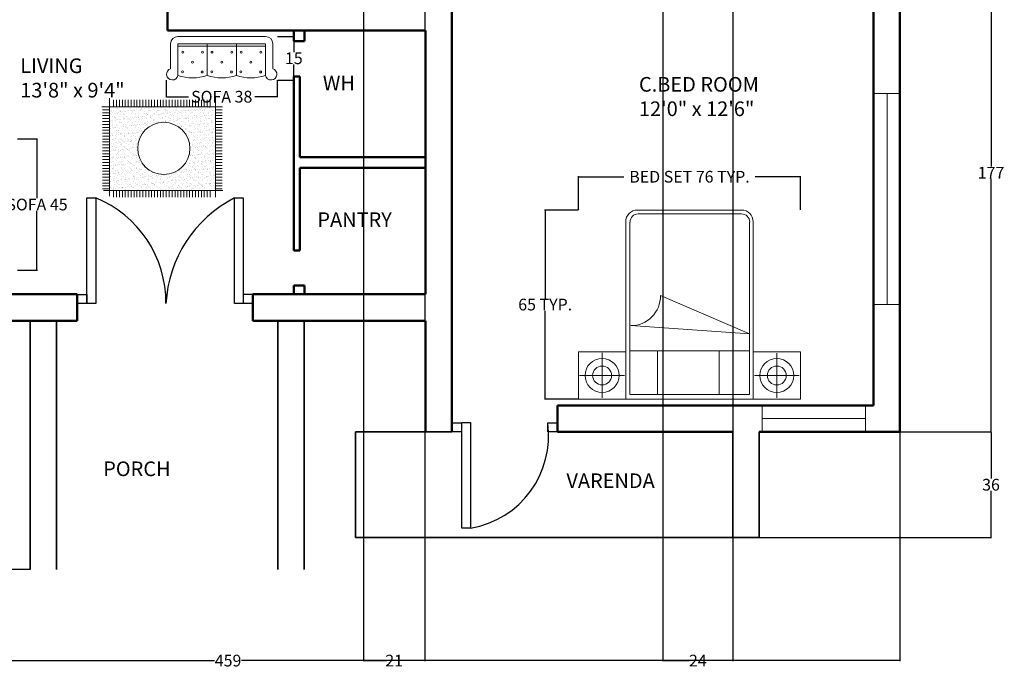
# Model space of a CAD drawing. Units: inches. Extents: x 870 to 1431, y 383 to 1070.
# Tile 2 of 9: x 1091 to 1428, y 383 to 604. Entities that reach past the tile are written whole.
import ezdxf
from ezdxf.lldxf.tags import DXFTag

# ---------------------------------------------------------------- set-up
doc = ezdxf.new("R2010")
doc.units = ezdxf.units.IN
doc.header["$MEASUREMENT"] = 0
for name, color, linetype, lineweight in [('A-ANNO-DIMS', 2, 'Continuous', 18), ('A-AREA-IDEN', 7, 'Continuous', 25), ('A-DOOR', 3, 'Continuous', 25), ('A-FLOR-EXTR', 7, 'Continuous', 35), ('A-FLOR-PATT', 252, 'Continuous', 13), ('A-FLOR-PORC', 7, 'HOT_WATER_SUPPLY', 35), ('A-FURN', 8, 'Continuous', 18), ('A-GLAZ', 4, 'Continuous', 18), ('A-WALL', 7, 'Continuous', 50)]:
    doc.layers.add(name, color=color, linetype=linetype, lineweight=lineweight)
doc.styles.get("Standard").update_dxf_attribs({"font": 'arial.ttf'})
tags = doc.linetypes.add('HOT_WATER_SUPPLY', pattern='A,0.5,-0.2,["HW",Standard,S=0.1,R=0,X=-0.1,Y=-0.05],-0.2', length=0.9).pattern_tags.tags
tags[6] = DXFTag(74, 10)
doc.dimstyles.get("Standard").update_dxf_attribs({"dimtxt": 4, "dimasz": 0.18, "dimexe": 0.18, "dimexo": 0.0625, "dimgap": 0.09, "dimtad": 0, "dimtih": 1, "dimtoh": 1, "dimdec": 0, "dimrnd": 6, "dimzin": 0, "dimdsep": 46, "dimlunit": 3, "dimtxsty": 'Standard', "dimcen": 0.09, "dimadec": 0, "dimazin": 0, "dimtfac": 1, "dimtdec": 0, "dimtofl": 0, "dimtmove": 0, "dimatfit": 3, "dimfxl": 1, "dimtolj": 1, "dimtzin": 0, "dimarcsym": 0})

# ---------------------------------------------------------------- blocks, each defined once
blk = doc.blocks.new('A$C65997121')
for p, q in [((0, 1.5, -0.169), (0, 2, -0.169)), ((0, 2, -0.169), (0.5, 2, -0.169)), ((0, 1.5, -0.169), (0, 2, -0.169)), ((0, 2, -0.169), (0.5, 2, -0.169)), ((0.25, 1.75, -0.169), (0.25, 1.988, -0.169)), ((0.5, 2, -0.169), (1.755, 2, -0.169)), ((0.5, 2, -0.169), (1.512, 2, -0.169)), ((0.5, 2, -0.169), (1.512, 2, -0.169)), ((0.5, 0.125, -0.169), (0.5, 2, -0.169)), ((0.5, 2, -0.169), (0.5, 1.5, -0.169)), ((1.512, 2, -0.169), (2.35, 2, -0.169)), ((1.512, 2, -0.169), (2.35, 2, -0.169)), ((1.85, 2, -0.169), (2.35, 2, -0.169)), ((1.85, 1.5, -0.169), (1.85, 2, -0.169)), ((2.1, 1.75, -0.169), (2.1, 1.988, -0.169)), ((2.35, 2, -0.169), (2.35, 1.5, -0.169)), ((2.35, 2, -0.169), (2.35, 1.5, -0.169)), ((2.35, 2, -0.169), (2.35, 1.5, -0.169)), ((0.538, 1.488, -0.169), (0.538, 1.952, -0.169)), ((0.538, 1.952, -0.169), (1.805, 1.952, -0.169)), ((0.86, 1.952, -0.169), (0.86, 1.488, -0.169)), ((1.512, 1.952, -0.169), (1.512, 1.488, -0.169)), ((1.805, 1.952, -0.169), (1.805, 1.488, -0.169)), ((0.25, 1.75, -0.169), (0.012, 1.75, -0.169)), ((0.25, 1.75, -0.169), (0.25, 1.512, -0.169)), ((0.25, 1.75, -0.169), (0.488, 1.75, -0.169)), ((2.1, 1.75, -0.169), (1.862, 1.75, -0.169)), ((2.1, 1.75, -0.169), (2.338, 1.75, -0.169)), ((2.1, 1.75, -0.169), (2.1, 1.512, -0.169)), ((0.5, 1.5, -0.169), (0, 1.5, -0.169)), ((0.5, 1.5, -0.169), (0, 1.5, -0.169)), ((0.5, 0.125, -0.169), (0.5, 1.5, -0.169)), ((1.805, 1.488, -0.169), (0.538, 1.488, -0.169)), ((0.538, 0.128, -0.169), (0.538, 1.488, -0.169)), ((1.805, 1.488, -0.169), (1.805, 0.128, -0.169)), ((2.35, 1.5, -0.169), (1.85, 1.5, -0.169)), ((2.35, 1.5, -0.169), (1.85, 1.5, -0.169)), ((1.85, 1.5, -0.169), (1.85, 0.125, -0.169)), ((2.35, 1.5, -0.169), (1.85, 1.5, -0.169)), ((1.85, 1.5, -0.169), (1.85, 0.125, -0.169)), ((1.483, 0.905, -0.506), (0.538, 1.31, -0.506)), ((0.538, 1.31, -0.506), (1.797, 1.222, -0.506)), ((1.717, 0.04, -0.169), (0.625, 0.04, -0.169)), ((1.725, 0, -0.169), (0.625, 0, -0.169)), ((1.725, 0, -0.169), (0.625, 0, -0.169))]:
    blk.add_line(p, q)
for centre, radius in [((0.25, 1.75, -0.169), 0.18), ((2.1, 1.75, -0.169), 0.18), ((0.25, 1.75, -0.169), 0.1), ((2.1, 1.75, -0.169), 0.1)]:
    blk.add_circle(centre, radius)
for centre, radius, start, end in [((1.793, 0.911, -0.506), 0.311, 89.3268, 181.1229), ((0.625, 0.125, -0.169), 0.125, 179.9939, 269.9939), ((0.625, 0.125, -0.169), 0.125, 179.9939, 269.9939), ((0.625, 0.128, -0.169), 0.0875, 179.9939, 269.9939), ((1.717, 0.128, -0.169), 0.0875, 269.9939, 359.9939), ((1.725, 0.125, -0.169), 0.125, 269.9939, 359.9939), ((1.725, 0.125, -0.169), 0.125, 269.9939, 359.9939)]:
    blk.add_arc(centre, radius, start, end)
blk = doc.blocks.new('A$C4BF50411')
for p, q in [((0.23, 0.89, -342.513), (2.03, 0.89, -342.513)), ((0.08, 0.74, -342.513), (0.08, 0.228, -342.513)), ((0.23, 0.09, -342.513), (0.23, 0.74, -342.513)), ((0.23, 0.74, -342.513), (2.03, 0.74, -342.513)), ((0.23, 0.69, -342.513), (2.03, 0.69, -342.513)), ((0.83, 0.09, -342.513), (0.83, 0.74, -342.513)), ((1.43, 0.74, -342.513), (1.43, 0.09, -342.513)), ((2.03, 0.74, -342.513), (2.03, 0.09, -342.513)), ((2.18, 0.74, -342.513), (2.18, 0.228, -342.513))]:
    blk.add_line(p, q)
for centre in [(0.33, 0.57, -342.513), (0.735, 0.565, -342.513), (0.93, 0.57, -342.513), (1.335, 0.565, -342.513), (1.53, 0.57, -342.513), (1.935, 0.565, -342.513), (0.53, 0.365, -342.513), (1.13, 0.365, -342.513), (1.73, 0.365, -342.513), (0.325, 0.165, -342.513), (0.73, 0.16, -342.513), (0.925, 0.165, -342.513), (1.33, 0.16, -342.513), (1.525, 0.165, -342.513), (1.93, 0.16, -342.513)]:
    blk.add_circle(centre, 0.02)
for centre, radius, start, end in [((0.23, 0.74, -342.513), 0.15, 90, 180), ((2.03, 0.74, -342.513), 0.15, 0, 90), ((0.115, 0.115, -342.513), 0.118, 107.205, 347.5934), ((2.145, 0.115, -342.513), 0.118, 192.4066, 72.795), ((0.53, 0.938, -342.513), 0.9, 250.5288, 289.4712), ((1.13, 0.938, -342.513), 0.9, 250.5288, 289.4712), ((1.73, 0.938, -342.513), 0.9, 250.5288, 289.4712)]:
    blk.add_arc(centre, radius, start, end)
blk = doc.blocks.new('WIN-72IN')
blk.add_line((4.72, 72), (4.72, 0))
blk.add_lwpolyline([(0, 72), (9, 72), (9, 0), (0, 0)], close=True)
blk = doc.blocks.new('WIN-BATH-35IN')
blk.add_line((4.73, 35.25), (4.73, 0))
blk.add_lwpolyline([(0, 0), (0, 35.25), (9, 35.25), (9, 0)], close=True)
blk = doc.blocks.new('*D107')
at = {"layer": 'A-ANNO-DIMS', "color": 0, "lineweight": -2, "transparency": 16777216}
for p, q in [((1282.02, 539.3), (1282.02, 550.79)), ((1282.2, 550.61), (1297.47, 550.61)), ((1357.67, 550.61), (1342.4, 550.61)), ((1357.85, 539.29), (1357.85, 550.79))]:
    blk.add_line(p, q, dxfattribs=at)
at = {"layer": 'A-ANNO-DIMS', "color": 0, "transparency": 16777216}
for points in [[(1282.2, 550.64), (1282.2, 550.58), (1282.02, 550.61)], [(1357.67, 550.64), (1357.67, 550.58), (1357.85, 550.61)]]:
    blk.add_solid(points, dxfattribs=at)
at = {"layer": 'Defpoints', "color": 0, "transparency": 16777216}
for p in [(1282.02, 550.61), (1282.02, 539.24), (1357.85, 539.23)]:
    blk.add_point(p, dxfattribs=at)
at = {"layer": 'A-ANNO-DIMS', "color": 0, "transparency": 16777216, "insert": (1319.94, 550.61), "char_height": 4, "attachment_point": 5}
blk.add_mtext('\\A1;BED SET 76 TYP.', dxfattribs=at)
blk = doc.blocks.new('*D108')
at = {"layer": 'A-ANNO-DIMS', "color": 0, "lineweight": -2, "transparency": 16777216}
for p, q in [((1281.96, 539.24), (1270.46, 539.24)), ((1270.64, 539.06), (1270.64, 509.1)), ((1270.64, 474.88), (1270.64, 504.84)), ((1281.95, 474.7), (1270.46, 474.7))]:
    blk.add_line(p, q, dxfattribs=at)
at = {"layer": 'A-ANNO-DIMS', "color": 0, "transparency": 16777216}
for points in [[(1270.61, 539.06), (1270.67, 539.06), (1270.64, 539.24)], [(1270.61, 474.88), (1270.67, 474.88), (1270.64, 474.7)]]:
    blk.add_solid(points, dxfattribs=at)
at = {"layer": 'Defpoints', "color": 0, "transparency": 16777216}
for p in [(1282.02, 539.24), (1270.64, 474.7), (1282.01, 474.7)]:
    blk.add_point(p, dxfattribs=at)
at = {"layer": 'A-ANNO-DIMS', "color": 0, "transparency": 16777216, "insert": (1270.64, 506.97), "char_height": 4, "attachment_point": 5}
blk.add_mtext('\\A1;65 TYP.', dxfattribs=at)
blk = doc.blocks.new('*D113')
at = {"layer": 'A-ANNO-DIMS', "color": 0, "lineweight": -2, "transparency": 16777216}
for p, q in [((1141.19, 583.55), (1141.19, 577.75)), ((1179.08, 583.55), (1179.08, 577.75)), ((1141.37, 577.93), (1148.8, 577.93)), ((1178.9, 577.93), (1171.47, 577.93))]:
    blk.add_line(p, q, dxfattribs=at)
at = {"layer": 'A-ANNO-DIMS', "color": 0, "transparency": 16777216}
for points in [[(1141.37, 577.96), (1141.37, 577.9), (1141.19, 577.93)], [(1178.9, 577.96), (1178.9, 577.9), (1179.08, 577.93)]]:
    blk.add_solid(points, dxfattribs=at)
at = {"layer": 'Defpoints', "color": 0, "transparency": 16777216}
for p in [(1141.19, 583.61), (1179.08, 583.61), (1179.08, 577.93)]:
    blk.add_point(p, dxfattribs=at)
at = {"layer": 'A-ANNO-DIMS', "color": 0, "transparency": 16777216, "insert": (1160.13, 577.93), "char_height": 4, "attachment_point": 5}
blk.add_mtext('\\A1;SOFA 38', dxfattribs=at)
blk = doc.blocks.new('*D114')
at = {"layer": 'A-ANNO-DIMS', "color": 0, "lineweight": -2, "transparency": 16777216}
for p, q in [((1179.14, 598.49), (1184.94, 598.49)), ((1184.76, 598.31), (1184.76, 593.18)), ((1184.76, 583.79), (1184.76, 588.92)), ((1179.14, 583.61), (1184.94, 583.61))]:
    blk.add_line(p, q, dxfattribs=at)
at = {"layer": 'A-ANNO-DIMS', "color": 0, "transparency": 16777216}
for points in [[(1184.73, 598.31), (1184.79, 598.31), (1184.76, 598.49)], [(1184.73, 583.79), (1184.79, 583.79), (1184.76, 583.61)]]:
    blk.add_solid(points, dxfattribs=at)
at = {"layer": 'Defpoints', "color": 0, "transparency": 16777216}
for p in [(1179.08, 598.49), (1184.76, 598.49), (1179.08, 583.61)]:
    blk.add_point(p, dxfattribs=at)
at = {"layer": 'A-ANNO-DIMS', "color": 0, "transparency": 16777216, "insert": (1184.76, 591.05), "char_height": 4, "attachment_point": 5}
blk.add_mtext('\\A1;15', dxfattribs=at)
blk = doc.blocks.new('*D115')
at = {"layer": 'A-ANNO-DIMS', "color": 0, "lineweight": -2, "transparency": 16777216}
for p, q in [((1090.35, 563.55), (1097.19, 563.55)), ((1097.01, 563.37), (1097.01, 543.29)), ((1097.01, 518.89), (1097.01, 538.97)), ((1090.35, 518.71), (1097.19, 518.71))]:
    blk.add_line(p, q, dxfattribs=at)
at = {"layer": 'A-ANNO-DIMS', "color": 0, "transparency": 16777216}
for points in [[(1096.98, 563.37), (1097.04, 563.37), (1097.01, 563.55)], [(1096.98, 518.89), (1097.04, 518.89), (1097.01, 518.71)]]:
    blk.add_solid(points, dxfattribs=at)
at = {"layer": 'Defpoints', "color": 0, "transparency": 16777216}
for p in [(1090.29, 563.55), (1097.01, 563.55), (1090.29, 518.71)]:
    blk.add_point(p, dxfattribs=at)
at = {"layer": 'A-ANNO-DIMS', "color": 0, "transparency": 16777216, "insert": (1097.01, 541.13), "char_height": 4, "attachment_point": 5}
blk.add_mtext('\\A1;SOFA 45', dxfattribs=at)
blk = doc.blocks.new('*D125')
at = {"layer": 'A-ANNO-DIMS', "color": 0, "lineweight": -2, "transparency": 16777216}
for p, q in [((1391.79, 463.41), (1391.79, 385.26)), ((932.79, 427.41), (932.79, 385.26)), ((932.97, 385.44), (1157.7, 385.44)), ((1391.61, 385.44), (1166.88, 385.44))]:
    blk.add_line(p, q, dxfattribs=at)
at = {"layer": 'A-ANNO-DIMS', "color": 0, "transparency": 16777216}
for points in [[(932.97, 385.47), (932.97, 385.41), (932.79, 385.44)], [(1391.61, 385.47), (1391.61, 385.41), (1391.79, 385.44)]]:
    blk.add_solid(points, dxfattribs=at)
at = {"layer": 'Defpoints', "color": 0, "transparency": 16777216}
for p in [(1391.79, 463.48), (932.79, 427.48), (1391.79, 385.44)]:
    blk.add_point(p, dxfattribs=at)
at = {"layer": 'A-ANNO-DIMS', "color": 0, "transparency": 16777216, "insert": (1162.29, 385.44), "char_height": 4, "attachment_point": 5}
blk.add_mtext('\\A1;459', dxfattribs=at)
blk = doc.blocks.new('*D126')
at = {"layer": 'A-ANNO-DIMS', "color": 0, "lineweight": -2, "transparency": 16777216}
for p, q in [((1168.73, 1009.48), (876.24, 1009.48)), ((876.42, 1009.3), (876.42, 715.17)), ((876.42, 416.77), (876.42, 710.9)), ((1094.63, 416.59), (876.24, 416.59))]:
    blk.add_line(p, q, dxfattribs=at)
at = {"layer": 'A-ANNO-DIMS', "color": 0, "transparency": 16777216}
for points in [[(876.39, 1009.3), (876.45, 1009.3), (876.42, 1009.48)], [(876.39, 416.77), (876.45, 416.77), (876.42, 416.59)]]:
    blk.add_solid(points, dxfattribs=at)
at = {"layer": 'Defpoints', "color": 0, "transparency": 16777216}
for p in [(876.42, 1009.48), (1168.79, 1009.48), (1094.7, 416.59)]:
    blk.add_point(p, dxfattribs=at)
at = {"layer": 'A-ANNO-DIMS', "color": 0, "transparency": 16777216, "insert": (876.42, 713.03), "char_height": 4, "attachment_point": 5}
blk.add_mtext('\\A1;592.9', dxfattribs=at)
blk = doc.blocks.new('*D134')
at = {"layer": 'A-ANNO-DIMS', "color": 0, "lineweight": -2, "transparency": 16777216}
for p, q in [((1391.85, 640.48), (1423.14, 640.48)), ((1422.96, 640.3), (1422.96, 554.08)), ((1422.96, 463.66), (1422.96, 549.88)), ((1391.85, 463.48), (1423.14, 463.48))]:
    blk.add_line(p, q, dxfattribs=at)
at = {"layer": 'A-ANNO-DIMS', "color": 0, "transparency": 16777216}
for points in [[(1422.93, 640.3), (1422.99, 640.3), (1422.96, 640.48)], [(1422.93, 463.66), (1422.99, 463.66), (1422.96, 463.48)]]:
    blk.add_solid(points, dxfattribs=at)
at = {"layer": 'Defpoints', "color": 0, "transparency": 16777216}
for p in [(1391.79, 640.48), (1391.79, 463.48), (1422.96, 463.48)]:
    blk.add_point(p, dxfattribs=at)
at = {"layer": 'A-ANNO-DIMS', "color": 0, "transparency": 16777216, "insert": (1422.96, 551.98), "char_height": 4, "attachment_point": 5}
blk.add_mtext('\\A1;177', dxfattribs=at)
blk = doc.blocks.new('*D135')
at = {"layer": 'A-ANNO-DIMS', "color": 0, "lineweight": -2, "transparency": 16777216}
for p, q in [((1343.85, 463.48), (1423.14, 463.48)), ((1422.96, 463.3), (1422.96, 447.61)), ((1422.96, 427.66), (1422.96, 443.34)), ((1343.85, 427.48), (1423.14, 427.48))]:
    blk.add_line(p, q, dxfattribs=at)
at = {"layer": 'A-ANNO-DIMS', "color": 0, "transparency": 16777216}
for points in [[(1422.93, 463.3), (1422.99, 463.3), (1422.96, 463.48)], [(1422.93, 427.66), (1422.99, 427.66), (1422.96, 427.48)]]:
    blk.add_solid(points, dxfattribs=at)
at = {"layer": 'Defpoints', "color": 0, "transparency": 16777216}
for p in [(1343.79, 463.48), (1422.96, 463.48), (1343.79, 427.48)]:
    blk.add_point(p, dxfattribs=at)
at = {"layer": 'A-ANNO-DIMS', "color": 0, "transparency": 16777216, "insert": (1422.96, 445.48), "char_height": 4, "attachment_point": 5}
blk.add_mtext('\\A1;36', dxfattribs=at)
blk = doc.blocks.new('*D136')
at = {"layer": 'A-ANNO-DIMS', "color": 0, "lineweight": -2, "transparency": 16777216}
for p, q in [((1208.53, 986.13), (1208.53, 385.26)), ((1229.53, 986.13), (1229.53, 385.26)), ((1208.71, 385.44), (1216.43, 385.44)), ((1229.35, 385.44), (1221.64, 385.44))]:
    blk.add_line(p, q, dxfattribs=at)
at = {"layer": 'A-ANNO-DIMS', "color": 0, "transparency": 16777216}
for points in [[(1208.71, 385.47), (1208.71, 385.41), (1208.53, 385.44)], [(1229.35, 385.47), (1229.35, 385.41), (1229.53, 385.44)]]:
    blk.add_solid(points, dxfattribs=at)
at = {"layer": 'Defpoints', "color": 0, "transparency": 16777216}
for p in [(1208.53, 986.19), (1229.53, 986.19), (1229.53, 385.44)]:
    blk.add_point(p, dxfattribs=at)
at = {"layer": 'A-ANNO-DIMS', "color": 0, "transparency": 16777216, "insert": (1219.03, 385.44), "char_height": 4, "attachment_point": 5}
blk.add_mtext('\\A1;21', dxfattribs=at)
blk = doc.blocks.new('*D141')
at = {"layer": 'A-ANNO-DIMS', "color": 0, "lineweight": -2, "transparency": 16777216}
for p, q in [((1310.79, 640.41), (1310.79, 385.26)), ((1334.79, 640.41), (1334.79, 385.26)), ((1310.97, 385.44), (1319.81, 385.44)), ((1334.61, 385.44), (1325.77, 385.44))]:
    blk.add_line(p, q, dxfattribs=at)
at = {"layer": 'A-ANNO-DIMS', "color": 0, "transparency": 16777216}
for points in [[(1310.97, 385.47), (1310.97, 385.41), (1310.79, 385.44)], [(1334.61, 385.47), (1334.61, 385.41), (1334.79, 385.44)]]:
    blk.add_solid(points, dxfattribs=at)
at = {"layer": 'Defpoints', "color": 0, "transparency": 16777216}
for p in [(1310.79, 640.48), (1334.79, 640.48), (1334.79, 385.44)]:
    blk.add_point(p, dxfattribs=at)
at = {"layer": 'A-ANNO-DIMS', "color": 0, "transparency": 16777216, "insert": (1322.79, 385.44), "char_height": 4, "attachment_point": 5}
blk.add_mtext('\\A1;24', dxfattribs=at)

msp = doc.modelspace()

# ---------------------------------------------------------------- hatches: boundary and pattern name
at = {"layer": 'A-FLOR-PATT'}
h = msp.add_hatch(dxfattribs=at)
h.set_pattern_fill('AR-SAND', color=256)
h.paths.add_polyline_path([(1157.9765, 574.4717), (1121.7456, 574.4717), (1121.7456, 545.9615), (1157.9765, 545.9615)])
h.paths.add_polyline_path([(1131.4117, 560.2829, -1), (1149.2393, 560.2829, -1)], flags=16)

# ---------------------------------------------------------------- linework, layer by layer
at = {"layer": 'A-DOOR'}
for p, q in [((1110.8005, 507.3667), (1110.8005, 510.4681)), ((1110.8005, 510.4681), (1114.0698, 510.4681)), ((1114.0698, 510.4681), (1114.0698, 507.3667)), ((1114.0698, 507.3667), (1110.8005, 507.3667))]:
    msp.add_line(p, q, dxfattribs=at)
for points in [[(1117.0698, 543.3667), (1117.0698, 507.3667), (1114.0698, 507.3667), (1114.0698, 543.3667)], [(1167.4988, 543.3667), (1167.4988, 507.3667), (1164.4988, 507.3667), (1164.4988, 543.3667)], [(1170.7907, 507.3759), (1167.5214, 507.3759), (1167.5214, 510.4772), (1170.7907, 510.4772)], [(1242.0601, 463.4772), (1238.7907, 463.4772), (1238.7907, 466.5786), (1242.0601, 466.5786)], [(1245.1554, 466.6646), (1245.1554, 430.6646), (1242.1554, 430.6646), (1242.1554, 466.6646)], [(1274.7907, 463.4772), (1271.5214, 463.4772), (1271.5214, 466.5786), (1274.7907, 466.5786)]]:
    msp.add_lwpolyline(points, close=True, dxfattribs=at)
for centre, radius, start, end in [((1102.5288, 507.6727), 38.5422, 359.545138, 67.834997), ((1183.9389, 505.0912), 42.9294, 116.925942, 176.961523), ((1239.8307, 462.2089), 31.9905, 279.581162, 7.850751)]:
    msp.add_arc(centre, radius, start, end, dxfattribs=at)
at = {"layer": 'A-FLOR-EXTR'}
for p, q in [((1205.7907, 463.4772), (1238.7907, 463.4772)), ((1205.7907, 463.4772), (1205.7907, 427.4772)), ((1334.7907, 463.4772), (1334.7907, 427.4772)), ((1343.7907, 463.4772), (1343.7907, 427.4772)), ((1205.7907, 427.4772), (1343.7907, 427.4772))]:
    msp.add_line(p, q, dxfattribs=at)
at = {"layer": 'A-FLOR-PORC', "ltscale": 15}
for p, q in [((1094.6967, 416.59), (1094.6967, 501.4772)), ((1103.6967, 416.59), (1103.6967, 501.4772)), ((1179.2821, 416.59), (1179.2821, 501.4772)), ((1188.2821, 416.59), (1188.2821, 501.4772))]:
    msp.add_line(p, q, dxfattribs=at)
at = {"layer": 'A-FURN'}
for p, q in [((1121.7456, 574.4717), (1121.7456, 577.4707)), ((1123.1675, 576.8165), (1123.1675, 574.4717)), ((1124.1675, 576.8165), (1124.1675, 574.4717)), ((1125.1675, 576.8165), (1125.1675, 574.4717)), ((1126.1675, 576.8165), (1126.1675, 574.4717)), ((1127.1675, 576.8165), (1127.1675, 574.4717)), ((1128.1675, 576.8165), (1128.1675, 574.4717)), ((1129.1675, 576.8165), (1129.1675, 574.4717)), ((1130.1675, 576.8165), (1130.1675, 574.4717)), ((1131.1675, 576.8165), (1131.1675, 574.4717)), ((1132.1675, 576.8165), (1132.1675, 574.4717)), ((1133.1675, 576.8165), (1133.1675, 574.4717)), ((1134.1675, 576.8165), (1134.1675, 574.4717)), ((1135.1675, 576.8165), (1135.1675, 574.4717)), ((1136.1675, 576.8165), (1136.1675, 574.4717)), ((1137.1675, 576.8165), (1137.1675, 574.4717)), ((1138.1675, 576.8165), (1138.1675, 574.4717)), ((1139.1675, 576.8165), (1139.1675, 574.4717)), ((1140.1675, 576.8165), (1140.1675, 574.4717)), ((1141.1675, 576.8165), (1141.1675, 574.4717)), ((1142.1675, 576.8165), (1142.1675, 574.4717)), ((1143.1675, 576.8165), (1143.1675, 574.4717)), ((1144.1675, 576.8165), (1144.1675, 574.4717)), ((1145.1675, 576.8165), (1145.1675, 574.4717)), ((1146.1675, 576.8165), (1146.1675, 574.4717)), ((1147.1675, 576.8165), (1147.1675, 574.4717)), ((1148.1675, 576.8165), (1148.1675, 574.4717)), ((1149.1675, 576.8165), (1149.1675, 574.4717)), ((1150.1675, 576.8165), (1150.1675, 574.4717)), ((1151.1675, 576.8165), (1151.1675, 574.4717)), ((1152.1675, 576.8165), (1152.1675, 574.4717)), ((1153.1675, 576.8165), (1153.1675, 574.4717)), ((1154.1675, 576.8165), (1154.1675, 574.4717)), ((1155.1675, 576.8165), (1155.1675, 574.4717)), ((1156.1675, 576.8165), (1156.1675, 574.4717)), ((1157.9765, 574.4717), (1157.9765, 577.8525)), ((1119.164, 574.4717), (1121.7456, 574.4717)), ((1119.4008, 573.4717), (1121.7456, 573.4717)), ((1119.4008, 572.4717), (1121.7456, 572.4717)), ((1157.9765, 574.4717), (1160.4268, 574.4717)), ((1157.9765, 574.4717), (1160.3213, 574.4717)), ((1157.9765, 573.4717), (1160.3213, 573.4717)), ((1157.9765, 572.4717), (1160.3213, 572.4717)), ((1119.4008, 571.4717), (1121.7456, 571.4717)), ((1119.4008, 570.4717), (1121.7456, 570.4717)), ((1119.4008, 569.4717), (1121.7456, 569.4717)), ((1157.9765, 571.4717), (1160.3213, 571.4717)), ((1157.9765, 570.4717), (1160.3213, 570.4717)), ((1157.9765, 569.4717), (1160.3213, 569.4717)), ((1119.4008, 568.4717), (1121.7456, 568.4717)), ((1119.4008, 567.4717), (1121.7456, 567.4717)), ((1119.4008, 566.4717), (1121.7456, 566.4717)), ((1119.4008, 565.4717), (1121.7456, 565.4717)), ((1157.9765, 568.4717), (1160.3213, 568.4717)), ((1157.9765, 567.4717), (1160.3213, 567.4717)), ((1157.9765, 566.4717), (1160.3213, 566.4717)), ((1157.9765, 565.4717), (1160.3213, 565.4717)), ((1119.4008, 564.4717), (1121.7456, 564.4717)), ((1119.4008, 563.4717), (1121.7456, 563.4717)), ((1119.4008, 562.4717), (1121.7456, 562.4717)), ((1157.9765, 564.4717), (1160.3213, 564.4717)), ((1157.9765, 563.4717), (1160.3213, 563.4717)), ((1157.9765, 562.4717), (1160.3213, 562.4717)), ((1119.4008, 561.4717), (1121.7456, 561.4717)), ((1119.4008, 560.4717), (1121.7456, 560.4717)), ((1119.4008, 559.4717), (1121.7456, 559.4717)), ((1119.4008, 558.4717), (1121.7456, 558.4717)), ((1157.9765, 561.4717), (1160.3213, 561.4717)), ((1157.9765, 560.4717), (1160.3213, 560.4717)), ((1157.9765, 559.4717), (1160.3213, 559.4717)), ((1157.9765, 558.4717), (1160.3213, 558.4717)), ((1119.4008, 557.4717), (1121.7456, 557.4717)), ((1119.4008, 556.4717), (1121.7456, 556.4717)), ((1119.4008, 555.4717), (1121.7456, 555.4717)), ((1157.9765, 557.4717), (1160.3213, 557.4717)), ((1157.9765, 556.4717), (1160.3213, 556.4717)), ((1157.9765, 555.4717), (1160.3213, 555.4717)), ((1119.4008, 554.4717), (1121.7456, 554.4717)), ((1119.4008, 553.4717), (1121.7456, 553.4717)), ((1119.4008, 552.4717), (1121.7456, 552.4717)), ((1157.9765, 554.4717), (1160.3213, 554.4717)), ((1157.9765, 553.4717), (1160.3213, 553.4717)), ((1157.9765, 552.4717), (1160.3213, 552.4717)), ((1119.4008, 551.4717), (1121.7456, 551.4717)), ((1119.4008, 550.4717), (1121.7456, 550.4717)), ((1119.4008, 549.4717), (1121.7456, 549.4717)), ((1119.4008, 548.4717), (1121.7456, 548.4717)), ((1157.9765, 551.4717), (1160.3213, 551.4717)), ((1157.9765, 550.4717), (1160.3213, 550.4717)), ((1157.9765, 549.4717), (1160.3213, 549.4717)), ((1157.9765, 548.4717), (1160.3213, 548.4717)), ((1119.4008, 547.4717), (1121.7456, 547.4717)), ((1119.4008, 546.4717), (1121.7456, 546.4717)), ((1121.7456, 545.9615), (1119.7386, 545.9615)), ((1121.7456, 545.9615), (1121.7456, 543.9822)), ((1123.1675, 545.9615), (1123.1675, 543.6167)), ((1124.1675, 545.9615), (1124.1675, 543.6167)), ((1125.1675, 545.9615), (1125.1675, 543.6167)), ((1126.1675, 545.9615), (1126.1675, 543.6167)), ((1127.1675, 545.9615), (1127.1675, 543.6167)), ((1128.1675, 545.9615), (1128.1675, 543.6167)), ((1129.1675, 545.9615), (1129.1675, 543.6167)), ((1130.1675, 545.9615), (1130.1675, 543.6167)), ((1131.1675, 545.9615), (1131.1675, 543.6167)), ((1132.1675, 545.9615), (1132.1675, 543.6167)), ((1133.1675, 545.9615), (1133.1675, 543.6167)), ((1134.1675, 545.9615), (1134.1675, 543.6167)), ((1135.1675, 545.9615), (1135.1675, 543.6167)), ((1136.1675, 545.9615), (1136.1675, 543.6167)), ((1137.1675, 545.9615), (1137.1675, 543.6167)), ((1138.1675, 545.9615), (1138.1675, 543.6167)), ((1139.1675, 545.9615), (1139.1675, 543.6167)), ((1140.1675, 545.9615), (1140.1675, 543.6167)), ((1141.1675, 545.9615), (1141.1675, 543.6167)), ((1142.1675, 545.9615), (1142.1675, 543.6167)), ((1143.1675, 545.9615), (1143.1675, 543.6167)), ((1144.1675, 545.9615), (1144.1675, 543.6167)), ((1145.1675, 545.9615), (1145.1675, 543.6167)), ((1146.1675, 545.9615), (1146.1675, 543.6167)), ((1147.1675, 545.9615), (1147.1675, 543.6167)), ((1148.1675, 545.9615), (1148.1675, 543.6167)), ((1149.1675, 545.9615), (1149.1675, 543.6167)), ((1150.1675, 545.9615), (1150.1675, 543.6167)), ((1151.1675, 545.9615), (1151.1675, 543.6167)), ((1152.1675, 545.9615), (1152.1675, 543.6167)), ((1153.1675, 545.9615), (1153.1675, 543.6167)), ((1154.1675, 545.9615), (1154.1675, 543.6167)), ((1155.1675, 545.9615), (1155.1675, 543.6167)), ((1156.1675, 545.9615), (1156.1675, 543.6167)), ((1157.9765, 547.4717), (1160.3213, 547.4717)), ((1157.9765, 546.4717), (1160.3213, 546.4717)), ((1157.9765, 545.9615), (1160.5313, 545.9615)), ((1157.9765, 545.9615), (1157.9765, 543.669))]:
    msp.add_line(p, q, dxfattribs=at)
msp.add_lwpolyline([(1121.7456, 574.4717), (1157.9765, 574.4717), (1157.9765, 545.9615), (1121.7456, 545.9615)], close=True, dxfattribs=at)
msp.add_circle((1140.3255, 560.2829), 8.9138, dxfattribs=at)
at = {"layer": 'A-WALL'}
for p, q in [((1391.7907, 640.4772), (1391.7907, 463.4772)), ((1382.7907, 631.4772), (1382.7907, 472.4772)), ((1141.5753, 609.4772), (1141.5753, 600.4772)), ((1238.7907, 609.4772), (1238.7907, 463.4772)), ((1141.5753, 600.4772), (1229.7907, 600.4772)), ((1184.7907, 600.4772), (1184.7907, 596.8772)), ((1188.3907, 600.4772), (1188.3907, 596.8772)), ((1229.7907, 600.4772), (1229.7907, 510.4772)), ((1184.7907, 596.8772), (1188.3907, 596.8772)), ((1184.7907, 584.8772), (1186.7907, 584.8772)), ((1184.7907, 584.8772), (1184.7907, 525.4772)), ((1186.7907, 584.8772), (1186.7907, 557.2772)), ((1186.7907, 557.2772), (1229.7907, 557.2772)), ((1186.7907, 553.6772), (1229.7907, 553.6772)), ((1186.7907, 553.6772), (1186.7907, 525.4772)), ((1184.7907, 525.4772), (1186.7907, 525.4772)), ((1184.7907, 513.4772), (1188.3907, 513.4772)), ((1184.7907, 513.4772), (1184.7907, 510.4772)), ((1188.3907, 513.4772), (1188.3907, 510.4772)), ((1072.7907, 510.4772), (1110.7907, 510.4772)), ((1110.7907, 510.4772), (1110.7907, 501.4772)), ((1170.7907, 510.4772), (1170.7907, 501.4772)), ((1170.7907, 510.4772), (1229.7907, 510.4772)), ((941.7907, 501.4772), (1110.7907, 501.4772)), ((1170.7907, 501.4772), (1229.7907, 501.4772)), ((1229.7907, 501.4772), (1229.7907, 463.4772)), ((1274.7907, 472.4772), (1382.7907, 472.4772)), ((1274.7907, 472.4772), (1274.7907, 463.4772)), ((1274.7907, 463.4772), (1334.7907, 463.4772)), ((1343.7907, 463.4772), (1391.7907, 463.4772))]:
    msp.add_line(p, q, dxfattribs=at)

# ---------------------------------------------------------------- block references
at = {"layer": 'A-FURN', "xscale": 16.6257473420345, "yscale": 16.6257473420345, "zscale": 16.6257473420345}
msp.add_blockref('A$C4BF50411', (1141.3441, 583.6983, 5694.5391), dxfattribs=at)
at = {"layer": 'A-FURN', "xscale": 32.26790700275002, "yscale": 32.26790700275002, "zscale": 32.26790700275002, "rotation": 179.993902596236}
msp.add_blockref('A$C65997121', (1357.8506, 539.2305, 5.4452), dxfattribs=at)
at = {"layer": 'A-GLAZ'}
msp.add_blockref('WIN-72IN', (1382.7165, 507.0388), dxfattribs=at)
at = {"layer": 'A-GLAZ', "rotation": 90.00000000000003}
msp.add_blockref('WIN-BATH-35IN', (1380.0638, 463.3692), dxfattribs=at)

# ---------------------------------------------------------------- texts
at = {"layer": 'A-AREA-IDEN', "char_height": 5, "attachment_point": 1}
for s, insert in [('LIVING\\P13\'8" x 9\'4"', (1091.3082, 590.9985)), ('WH', (1194.6726, 585.126)), ('C.BED ROOM\\P12\'0" x 12\'6"', (1302.6771, 584.6527)), ('PANTRY', (1192.8044, 538.4583)), ('PORCH', (1119.627, 453.4108)), ('VARENDA', (1277.8908, 449.3379))]:
    msp.add_mtext_dynamic_manual_height_columns(s, width=69.132678, gutter_width=1, heights=[0], dxfattribs=dict(at, insert=insert))

# ---------------------------------------------------------------- dimensions: what is measured, and where the dimension line sits
at = {"layer": 'A-ANNO-DIMS'}
for base, p1, p2, override, picture, middle in [((876.4215, 1009.4772), (1094.6967, 416.59), (1168.7907, 1009.4772), {"dimdec": 1, "dimlfac": 1, "dimrnd": 0, "dimzin": 0, "dimdsep": 46, "dimlunit": 2}, '*D126', (876.4215, 713.0336)), ((1422.9581, 463.4772), (1391.7907, 640.4772), (1391.7907, 463.4772), {"dimdec": 0, "dimlfac": 1, "dimrnd": 0, "dimzin": 0, "dimdsep": 46, "dimlunit": 2}, '*D134', (1422.9581, 551.9772)), ((1184.759, 598.4909), (1179.0762, 583.6112), (1179.0762, 598.4909), {"dimdec": 0, "dimlfac": 1, "dimrnd": 0, "dimzin": 0, "dimdsep": 46, "dimlunit": 2}, '*D114', (1184.759, 591.0511)), ((1422.9581, 463.4772), (1343.7907, 427.4772), (1343.7907, 463.4772), {"dimdec": 0, "dimlfac": 1, "dimrnd": 0, "dimzin": 0, "dimdsep": 46, "dimlunit": 2}, '*D135', (1422.9581, 445.4772))]:
    dim = msp.add_linear_dim(base=base, p1=p1, p2=p2, angle=90, dimstyle='Standard', override=override, dxfattribs=at)
    dim.commit()
    dim.dimension.update_dxf_attribs({"geometry": picture, "text_midpoint": middle})
for base, p1, p2, picture, middle in [((1229.5328, 385.44), (1208.5328, 986.1907), (1229.5328, 986.1907), '*D136', (1219.0328, 385.44)), ((1334.7907, 385.44), (1310.7907, 640.4772), (1334.7907, 640.4772), '*D141', (1322.7907, 385.44)), ((1391.7907, 385.44), (932.7907, 427.4772), (1391.7907, 463.4772), '*D125', (1162.2907, 385.44))]:
    dim = msp.add_linear_dim(base=base, p1=p1, p2=p2, dimstyle='Standard', override={"dimdec": 0, "dimlfac": 1, "dimrnd": 0, "dimzin": 0, "dimdsep": 46, "dimlunit": 2}, dxfattribs=at)
    dim.commit()
    dim.dimension.update_dxf_attribs({"geometry": picture, "text_midpoint": middle})
dim = msp.add_linear_dim(base=(1179.0762, 577.9284), p1=(1141.1905, 583.6112), p2=(1179.0762, 583.6112), text='SOFA <>', dimstyle='Standard', override={"dimdec": 0, "dimlfac": 1, "dimrnd": 0, "dimzin": 0, "dimdsep": 46, "dimlunit": 2}, dxfattribs=at)
dim.commit()
dim.dimension.update_dxf_attribs({"geometry": '*D113', "text_midpoint": (1160.1333, 577.9284)})
for base, p1, p2, angle, text, picture, middle in [((1097.0146, 563.5502), (1090.2878, 518.7052), (1090.2878, 563.5502), 90, 'SOFA <>', '*D115', (1097.0146, 541.1277)), ((1282.0206, 550.6135), (1357.8506, 539.2307), (1282.0193, 539.2388), 179.993903, 'BED SET <> TYP.', '*D107', (1319.9362, 550.6094)), ((1270.6378, 474.6975), (1282.0193, 539.2388), (1282.0125, 474.6963), 269.993903, '<> TYP.', '*D108', (1270.6412, 506.9687))]:
    dim = msp.add_linear_dim(base=base, p1=p1, p2=p2, angle=angle, text=text, dimstyle='Standard', override={"dimdec": 0, "dimlfac": 1, "dimrnd": 0, "dimzin": 0, "dimdsep": 46, "dimlunit": 2}, dxfattribs=at)
    dim.commit()
    dim.dimension.update_dxf_attribs({"geometry": picture, "text_midpoint": middle})

doc.saveas('drawing.dxf')
